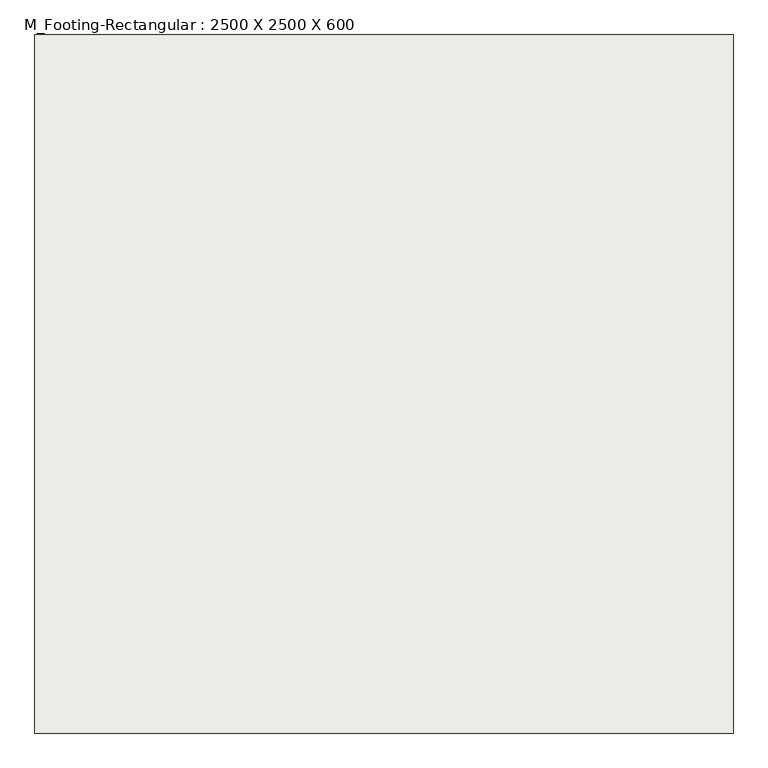
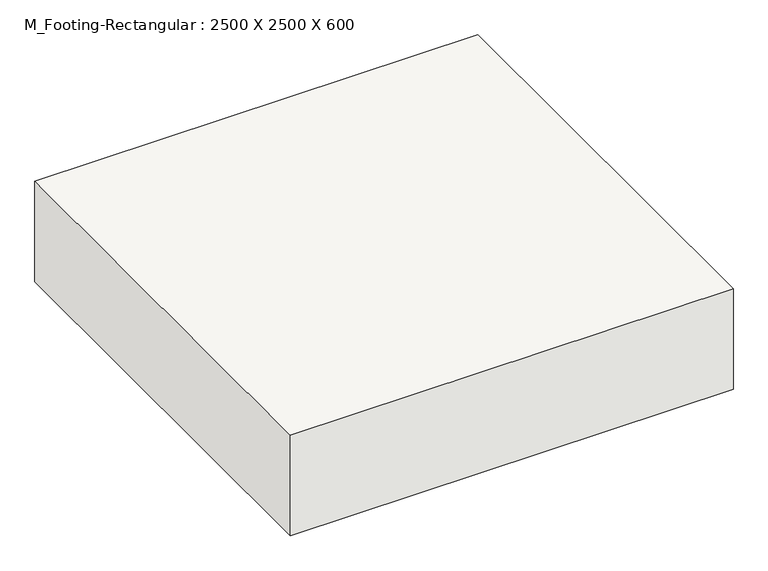
"""IFC4 building model written with IfcOpenShell, lengths in millimetres: slab geometry, M_Footing-Rectangular : 2500 X 2500 X 600."""

from ifc_helpers import new_model, si_unit, frame, origin, place, context, project, spatial, polyline, outline, extrude, source, transform, mapped, element, save


def m_footing_rectangular_2500_x_2500_x_600_5d9c2050(model_context):
    return source(origin(), model_context, "Body", "SweptSolid", [
        extrude(outline(polyline([(1250.0, 1250.0), (1250.0, -1250.0), (-1250.0, -1250.0), (-1250.0, 1250.0), (1250.0, 1250.0)])), frame((0.0, 0.0, -600.0), z_axis=(0.0, 0.0, 1.0), x_axis=(1.0, 0.0, 0.0)), (0.0, 0.0, 1.0), 600.0),
    ])


if __name__ == "__main__":
    model = new_model("IFC4")
    model_context = context("Model", 3, world=origin())
    ifc_project = project(units=[si_unit("LENGTHUNIT", "METRE", prefix="MILLI")], contexts=[model_context])
    site = spatial("IfcSite", under=ifc_project)
    building = spatial("IfcBuilding", under=site)
    placement = place(None, origin())
    m_footing_rectangular_2500_x_2500_x_600_shape = m_footing_rectangular_2500_x_2500_x_600_5d9c2050(model_context)
    element("IfcSlab", 1, ObjectType="M_Footing-Rectangular : 2500 X 2500 X 600", at=placement, inside=building, context=model_context, shape_type="MappedRepresentation", body=[
        mapped(m_footing_rectangular_2500_x_2500_x_600_shape, transform((0.0, 0.0, 0.0), x_axis=(1.0, 0.0, 0.0), y_axis=(0.0, 1.0, 0.0), z_axis=(0.0, 0.0, 1.0))),
    ])
    save(model, "model.ifc")

# Revit data of these elements
# Type "M_Footing-Rectangular : 2500 X 2500 X 600"
#   Width = 2500 mm
#   Length = 2500 mm
#   Foundation Thickness = 600 mm
#   Structural Material [instance default] = Concrete, Cast-in-Place gray
#   Assembly Code = ""
# Element 1 (IfcSlab, "M_Footing-Rectangular : 2500 X 2500 X 600")
#   Materials on its faces: "Concrete, Cast-in-Place gray"
# Materials
#   "Concrete, Cast-in-Place gray": class "Concrete", colour RGB 192 192 192, transparency 0, Description = "Cast-in-place concrete", Cost = 0
